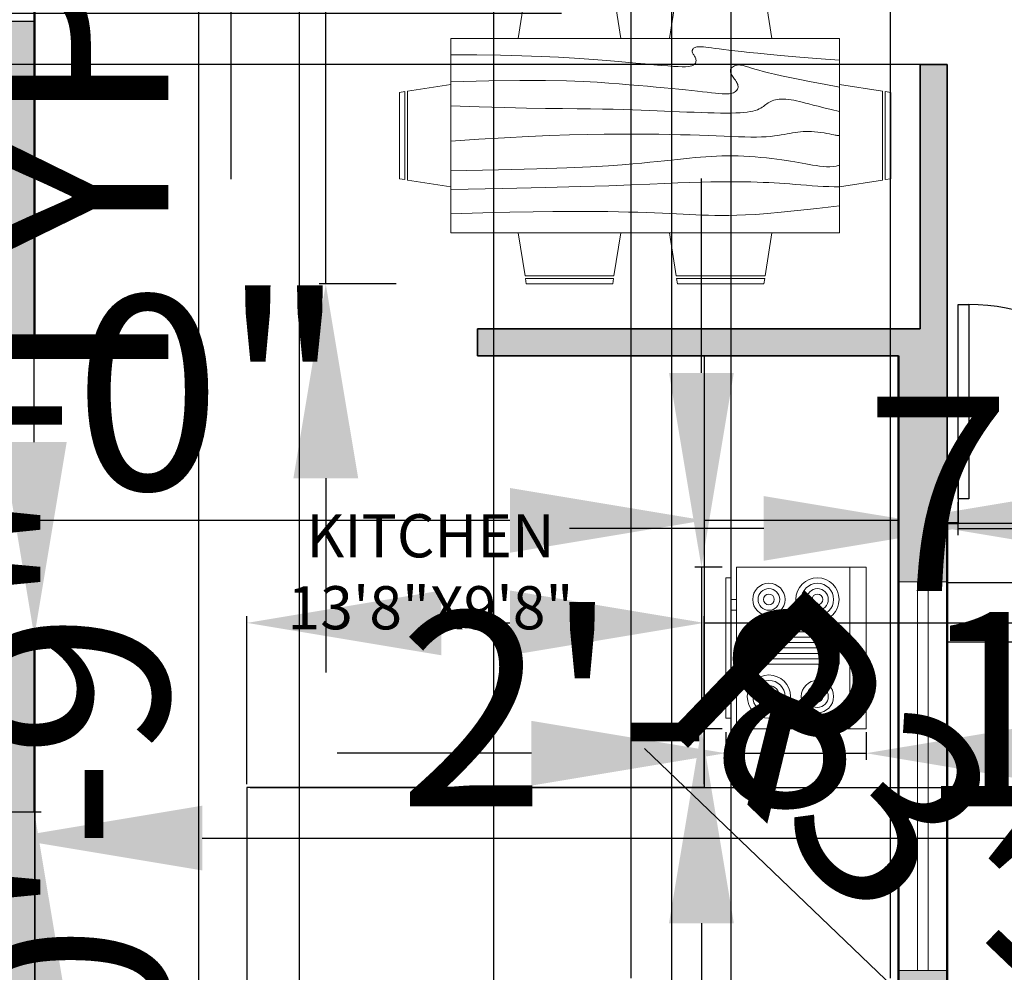
# Model space of a CAD drawing. Units: inches. Extents: x -299 to 1164, y -2 to 940.
# Tile 5 of 11: x 414 to 597, y 313 to 490. Entities that reach past the tile are written whole.
import ezdxf

# ---------------------------------------------------------------- set-up
doc = ezdxf.new("R2010")
doc.units = ezdxf.units.IN
for name, color, linetype, lineweight in [('A-AREA-IDEN', 3, 'Continuous', 25), ('A-EQPM', 8, 'Continuous', 18), ('A-FLOR-CASE', 7, 'Continuous', 25), ('A-FURN', 8, 'Continuous', 18), ('dimensions', 191, 'Continuous', 18), ('doors', 20, 'Continuous', 25), ('inner walls', 7, 'Continuous', 35), ('outer walls', 7, 'Continuous', 50), ('stairs', 6, 'Continuous', 25), ('windows', 130, 'Continuous', 18)]:
    doc.layers.add(name, color=color, linetype=linetype, lineweight=lineweight)
doc.layers.add('A-WALL-PATT', color=240, linetype='Continuous', lineweight=13, true_color=0xed1f24)
doc.styles.get("Standard").update_dxf_attribs({"font": 'arial.ttf'})
doc.dimstyles.new('ISO-25', dxfattribs={"dimtxt": 36, "dimasz": 36, "dimexe": 1.25, "dimexo": 0.625, "dimtad": 1, "dimlunit": 3, "dimtxsty": 'Standard', "dimcen": 2.5, "dimazin": 0, "dimtfac": 1, "dimtmove": 0, "dimatfit": 3, "dimfxl": 1, "dimarcsym": 0})

# ---------------------------------------------------------------- blocks, each defined once
blk = doc.blocks.new('Dining Set - 36 x 72 in.')
for p, q in [((-22, 27.5), (-22.1562, 26.50042)), ((-22, 27.5), (-6, 27.5)), ((-5.8437, 26.49966), (-6, 27.5)), ((6, 27.5), (5.8438, 26.50042)), ((6, 27.5), (22, 27.5)), ((22.1563, 26.49966), (22, 27.5)), ((-22.2343, 26.00059), (-23.4847, 17.99762)), ((-22.2304, 26), (-5.7608, 26)), ((-5.8416, 26.5), (-22.1534, 26.5)), ((-4.5152, 17.99762), (-5.7655, 25.99926)), ((5.7657, 26.00059), (4.5153, 17.99762)), ((5.7696, 26), (22.2392, 26)), ((22.1584, 26.5), (5.8466, 26.5)), ((23.4848, 17.99762), (22.2345, 25.99926)), ((36, 18), (-36, 18)), ((-36, 18), (-36, -18)), ((36, -18), (36, 18)), ((-44.0006, 8.23428), (-35.9976, 9.48474)), ((44.0006, 8.23428), (35.9976, 9.48474)), ((-45.5, 8), (-44.5004, 8.15617)), ((-45.5, 8), (-45.5, -8)), ((-44.5, -8.15843), (-44.5, 8.15338)), ((-44, 8.23041), (-44, -8.23915)), ((44, 8.23041), (44, -8.23915)), ((44.5, -8.15843), (44.5, 8.15338)), ((45.5, 8), (44.5005, 8.15617)), ((45.5, 8), (45.5, -8)), ((-44.4997, -8.15631), (-45.5, -8)), ((-35.9976, -9.48476), (-43.9993, -8.2345)), ((35.9976, -9.48476), (43.9993, -8.2345)), ((44.4997, -8.15631), (45.5, -8)), ((-36, -18), (36, -18)), ((-22.2343, -26.0006), (-23.4847, -17.99762)), ((-4.5152, -17.99762), (-5.7655, -25.99928)), ((5.7657, -26.0006), (4.5153, -17.99762)), ((23.4848, -17.99762), (22.2345, -25.99928)), ((-22.2304, -26), (-5.7608, -26)), ((-22, -27.5), (-22.1562, -26.50044)), ((-5.8416, -26.5), (-22.1534, -26.5)), ((-5.8437, -26.49967), (-6, -27.5)), ((5.7696, -26), (22.2392, -26)), ((6, -27.5), (5.8438, -26.50044)), ((22.1584, -26.5), (5.8466, -26.5)), ((22.1563, -26.49967), (22, -27.5)), ((-22, -27.5), (-6, -27.5)), ((6, -27.5), (22, -27.5))]:
    blk.add_line(p, q)
for points in [[(-36, 15), (-31.1772, 14.97754), (-26.8079, 14.91406), (-22.8538, 14.81543), (-19.276, 14.6875), (-16.0362, 14.53613), (-13.0957, 14.36718), (-10.4159, 14.18652), (-7.9583, 14), (-5.6904, 13.81315), (-3.6035, 13.63021), (-1.6954, 13.45508), (0.0365, 13.29166), (1.5945, 13.14388), (2.9811, 13.01562), (4.1988, 12.9108), (5.25, 12.83333), (6.1393, 12.78613), (6.8802, 12.76823), (7.4883, 12.77767), (7.9792, 12.8125), (8.3685, 12.87077), (8.6719, 12.95052), (8.9049, 13.0498), (9.0833, 13.16666), (9.2205, 13.29899), (9.3216, 13.44401), (9.3895, 13.59879), (9.4271, 13.76041), (9.4373, 13.92594), (9.4232, 14.09245), (9.3875, 14.257), (9.3333, 14.41666), (9.2638, 14.56917), (9.1836, 14.71484), (9.0975, 14.85465), (9.0104, 14.98958), (8.9272, 15.1206), (8.8529, 15.2487), (8.7922, 15.37483), (8.75, 15.5), (8.7305, 15.62467), (8.7344, 15.74739), (8.7617, 15.86621), (8.8125, 15.97916), (8.8867, 16.08431), (8.9844, 16.17968), (9.1055, 16.26334), (9.25, 16.33333), (9.4189, 16.38802), (9.6172, 16.42708), (9.8506, 16.45052), (10.125, 16.45833), (10.4463, 16.45052), (10.8203, 16.42708), (11.2529, 16.38802), (11.75, 16.33333), (12.3184, 16.26318), (12.9694, 16.17838), (13.7151, 16.07991), (14.5677, 15.96875), (15.5395, 15.84586), (16.6426, 15.71224), (17.8893, 15.56884), (19.2917, 15.41666), (20.859, 15.25667), (22.5879, 15.08984), (24.4721, 14.91715), (26.5052, 14.73958), (28.6809, 14.5581), (30.9929, 14.3737), (33.4347, 14.18733), (36, 14)], [(-36, 10), (-28.9766, 10.14274), (-23.1725, 10.20442), (-18.4241, 10.19775), (-14.5677, 10.13541), (-11.4399, 10.03011), (-8.877, 9.89453), (-6.7154, 9.74137), (-4.7917, 9.58333), (-2.9698, 9.43082), (-1.2246, 9.28515), (0.4415, 9.14534), (2.026, 9.01041), (3.5266, 8.87939), (4.9408, 8.7513), (6.266, 8.62516), (7.5, 8.5), (8.6411, 8.37549), (9.6914, 8.2539), (10.6538, 8.13818), (11.5312, 8.03125), (12.3267, 7.93603), (13.043, 7.85547), (13.6831, 7.79248), (14.25, 7.75), (14.7471, 7.7303), (15.1797, 7.73307), (15.5537, 7.75732), (15.875, 7.80208), (16.1494, 7.86637), (16.3828, 7.94922), (16.5811, 8.04964), (16.75, 8.16666), (16.8944, 8.29915), (17.0143, 8.44531), (17.1089, 8.60319), (17.1771, 8.77083), (17.218, 8.94629), (17.2305, 9.1276), (17.2137, 9.31282), (17.1667, 9.5), (17.0895, 9.6875), (16.987, 9.875), (16.8649, 10.0625), (16.7292, 10.25), (16.5856, 10.4375), (16.4401, 10.625), (16.2985, 10.8125), (16.1667, 11), (16.05, 11.18733), (15.9518, 11.3737), (15.8752, 11.5581), (15.8229, 11.73958), (15.798, 11.91715), (15.8034, 12.08984), (15.842, 12.25667), (15.9167, 12.41666), (16.0295, 12.56836), (16.1784, 12.70833), (16.3605, 12.83268), (16.5729, 12.9375), (16.8127, 13.01888), (17.0768, 13.07291), (17.3625, 13.0957), (17.6667, 13.08333), (17.9894, 13.03312), (18.3418, 12.94726), (18.7382, 12.82918), (19.1927, 12.68229), (19.7195, 12.51001), (20.3327, 12.31575), (21.0465, 12.10294), (21.875, 11.875), (22.8357, 11.63354), (23.959, 11.37304), (25.2786, 11.08618), (26.8282, 10.76562), (28.6414, 10.40405), (30.752, 9.99414), (33.1936, 9.52856), (36, 9)], [(-36, 5.5), (-30.7157, 5.3348), (-26.069, 5.20963), (-21.9946, 5.11767), (-18.4271, 5.05208), (-15.3009, 5.00602), (-12.5508, 4.97265), (-10.1112, 4.94515), (-7.9167, 4.91666), (-5.909, 4.88167), (-4.0586, 4.83984), (-2.3429, 4.79215), (-0.7396, 4.73958), (0.7739, 4.6831), (2.22, 4.6237), (3.6213, 4.56233), (5, 4.5), (6.373, 4.43782), (7.7344, 4.3776), (9.0723, 4.32129), (10.375, 4.27083), (11.6309, 4.22819), (12.8281, 4.19531), (13.9551, 4.17415), (15, 4.16666), (15.954, 4.17448), (16.819, 4.19791), (17.6001, 4.23698), (18.3021, 4.29166), (18.9299, 4.36198), (19.4883, 4.44791), (19.9823, 4.54948), (20.4167, 4.66666), (20.7969, 4.79899), (21.1302, 4.94401), (21.4245, 5.09879), (21.6875, 5.26041), (21.9271, 5.42594), (22.1511, 5.59245), (22.3672, 5.757), (22.5834, 5.91666), (22.8065, 6.06868), (23.0404, 6.21093), (23.2879, 6.34147), (23.5521, 6.45833), (23.8358, 6.55957), (24.142, 6.64323), (24.4735, 6.70735), (24.8334, 6.75), (25.2235, 6.76969), (25.642, 6.76692), (26.0858, 6.74267), (26.5521, 6.69791), (27.0379, 6.63362), (27.5404, 6.55078), (28.0565, 6.45036), (28.5834, 6.33333), (29.1242, 6.19987), (29.7071, 6.04687), (30.3661, 5.87044), (31.1354, 5.66666), (32.0493, 5.43164), (33.142, 5.16146), (34.4475, 4.85221), (36, 4.5)], [(-36, -1), (-30.7915, -0.6591), (-26.0195, -0.38216), (-21.6519, -0.16284), (-17.6563, 0.00521), (-14.0005, 0.12833), (-10.6523, 0.21289), (-7.5796, 0.26522), (-4.75, 0.29166), (-2.134, 0.29793), (0.2878, 0.28711), (2.5317, 0.26163), (4.6146, 0.22396), (6.5529, 0.17651), (8.3633, 0.12174), (10.0623, 0.06209), (11.6667, 0), (13.1899, -0.06201), (14.6341, -0.1211), (15.9982, -0.17432), (17.2813, -0.21875), (18.4823, -0.25147), (19.6003, -0.26953), (20.6343, -0.27002), (21.5834, -0.25), (22.4481, -0.20768), (23.2357, -0.14584), (23.9549, -0.06836), (24.6146, 0.02083), (25.2235, 0.11784), (25.7904, 0.21875), (26.3241, 0.31966), (26.8334, 0.41666), (27.3265, 0.50618), (27.8099, 0.58593), (28.2894, 0.65397), (28.7709, 0.70833), (29.2601, 0.74707), (29.763, 0.76823), (30.2855, 0.76985), (30.8334, 0.75), (31.4088, 0.70784), (31.9994, 0.64713), (32.589, 0.57275), (33.1615, 0.48958), (33.7008, 0.4025), (34.1908, 0.3164), (34.6153, 0.23616), (34.9584, 0.16666), (35.2099, 0.11165), (35.3848, 0.07031), (35.504, 0.04069), (35.5886, 0.02083), (35.6594, 0.00879), (35.7377, 0.0026), (35.8442, 0.00032), (36, 0)], [(-36, -6.5), (-27.1843, -6.31267), (-20.084, -6.1263), (-14.469, -5.9419), (-10.1094, -5.76042), (-6.7752, -5.58285), (-4.2363, -5.41016), (-2.2629, -5.24333), (-0.625, -5.08334), (0.8708, -4.93099), (2.2715, -4.78646), (3.5872, -4.64974), (4.8281, -4.52084), (6.0046, -4.39974), (7.127, -4.28646), (8.2053, -4.18099), (9.25, -4.08334), (10.2705, -3.99382), (11.2734, -3.91407), (12.2647, -3.84603), (13.25, -3.79167), (14.2354, -3.75293), (15.2266, -3.73177), (16.2295, -3.73015), (17.25, -3.75), (18.2912, -3.79248), (19.3451, -3.85547), (20.4009, -3.93604), (21.4479, -4.03125), (22.4754, -4.13819), (23.4727, -4.25391), (24.4289, -4.37549), (25.3334, -4.5), (26.1785, -4.62492), (26.9694, -4.74935), (27.7145, -4.87281), (28.4219, -4.99479), (29.1, -5.11483), (29.7572, -5.23242), (30.4016, -5.34709), (31.0417, -5.45834), (31.6837, -5.56437), (32.3262, -5.65821), (32.9658, -5.73153), (33.599, -5.77604), (34.2224, -5.78345), (34.8327, -5.74545), (35.4264, -5.65373), (36, -5.5)], [(-36, -10), (-26.4022, -9.81299), (-18.4675, -9.62891), (-11.9839, -9.45069), (-6.7396, -9.28125), (-2.5226, -9.12354), (0.8789, -8.98047), (3.6769, -8.85498), (6.0833, -8.75), (8.2767, -8.66765), (10.3021, -8.60677), (12.1712, -8.56543), (13.8958, -8.54167), (15.4876, -8.53353), (16.9583, -8.53907), (18.3197, -8.55632), (19.5834, -8.58334), (20.7616, -8.61841), (21.8685, -8.66081), (22.9188, -8.71004), (23.9271, -8.76563), (24.9081, -8.82707), (25.8763, -8.89388), (26.8465, -8.96558), (27.8334, -9.04167), (28.8474, -9.12118), (29.8828, -9.20117), (30.93, -9.27824), (31.9792, -9.34896), (33.0205, -9.40991), (34.0443, -9.45768), (35.0407, -9.48885), (36, -9.5)], [(-36, -14.5), (-30.0881, -14.33513), (-25.0332, -14.21224), (-20.7312, -14.12647), (-17.0781, -14.07292), (-13.97, -14.04671), (-11.3027, -14.04297), (-8.9724, -14.05681), (-6.875, -14.08334), (-4.9224, -14.11833), (-3.0905, -14.16016), (-1.3709, -14.20785), (0.2448, -14.26042), (1.7647, -14.3169), (3.1973, -14.3763), (4.5507, -14.43767), (5.8333, -14.5), (7.0554, -14.5621), (8.235, -14.62175), (9.3922, -14.67652), (10.5469, -14.72396), (11.7192, -14.76164), (12.929, -14.78711), (14.1965, -14.79794), (15.5417, -14.79167), (16.9933, -14.76424), (18.6152, -14.70508), (20.4804, -14.60197), (22.6615, -14.44271), (25.2312, -14.21509), (28.2624, -13.9069), (31.8277, -13.50594), (36, -13)]]:
    blk.add_lwpolyline(points)
blk = doc.blocks.new('Range-Oven - 30 in top')
for p, q in [((0, -3), (30, -3)), ((12, -6), (18, -6)), ((13, -20), (13, -6)), ((14, -6), (14, -20)), ((15, -20), (15, -6)), ((16, -6), (16, -20)), ((17, -20), (17, -6)), ((18, -20), (12, -20)), ((6, -24), (6, -25)), ((8, -25), (8, -24)), ((22, -25), (22, -24)), ((24, -24), (24, -25))]:
    blk.add_line(p, q)
for points in [[(0, -24), (0, 0), (30, 0), (30, -24)], [(12, -21), (12, -5), (18, -5), (18, -21)], [(2, -26), (2, -25), (28, -25), (28, -26)]]:
    blk.add_lwpolyline(points, close=True)
for centre, radius in [((6, -9), 4), ((6, -9), 3), ((6, -9), 2), ((24, -9), 3), ((24, -9), 2), ((6, -9), 1), ((24, -9), 1), ((24, -18), 4), ((6, -18), 3), ((6, -18), 2), ((24, -18), 3), ((24, -18), 2), ((6, -18), 1), ((24, -18), 1)]:
    blk.add_circle(centre, radius)
blk = doc.blocks.new('WIN-72IN')
for p, q in [((0, 5.5), (72, 5.5)), ((0, 3.5), (72, 3.5))]:
    blk.add_line(p, q)
blk.add_lwpolyline([(0, 0), (72, 0), (72, 9), (0, 9)], close=True)
blk = doc.blocks.new('DOOR-36IN')
blk.add_lwpolyline([(0, 36), (2, 36), (2, 0), (0, 0)], close=True)
blk.add_arc((2.32, 2.25), 33.75, 356.1776, 90.5492)
blk = doc.blocks.new('*D25')
at = {"layer": 'Defpoints', "color": 0, "transparency": 16777216}
for p in [(443.65, 597.1), (453.38, 597.1), (443.65, 532.21)]:
    blk.add_point(p, dxfattribs=at)
at = {"layer": 'dimensions', "color": 0, "lineweight": -2, "transparency": 16777216}
for p, q in [((453.38, 633.1), (453.38, 916.77)), ((444.27, 597.1), (454.63, 597.1)), ((453.38, 532.21), (453.38, 597.1)), ((444.27, 532.21), (454.63, 532.21)), ((453.38, 496.21), (453.38, 460.21))]:
    blk.add_line(p, q, dxfattribs=at)
at = {"layer": 'dimensions', "color": 0, "transparency": 16777216}
for points in [[(447.38, 633.1), (459.38, 633.1), (453.38, 597.1)], [(447.38, 496.21), (459.38, 496.21), (453.38, 532.21)]]:
    blk.add_solid(points, dxfattribs=at)
at = {"layer": 'dimensions', "color": 0, "transparency": 16777216, "insert": (434.13, 792.94), "char_height": 36, "attachment_point": 5, "rotation": 90}
blk.add_mtext('SOFA 5\'-5"', dxfattribs=at)
blk = doc.blocks.new('*D27')
at = {"layer": 'Defpoints', "color": 0, "transparency": 16777216}
for p in [(412.07, 375.49), (416.95, 375.49), (412.07, 342.99)]:
    blk.add_point(p, dxfattribs=at)
at = {"layer": 'dimensions', "color": 0, "lineweight": -2, "transparency": 16777216}
for p, q in [((416.95, 411.49), (416.95, 915.12)), ((412.7, 375.49), (418.2, 375.49)), ((416.95, 342.99), (416.95, 375.49)), ((412.7, 342.99), (418.2, 342.99)), ((416.95, 306.99), (416.95, 270.99))]:
    blk.add_line(p, q, dxfattribs=at)
at = {"layer": 'dimensions', "color": 0, "transparency": 16777216}
for points in [[(410.95, 411.49), (422.95, 411.49), (416.95, 375.49)], [(410.95, 306.99), (422.95, 306.99), (416.95, 342.99)]]:
    blk.add_solid(points, dxfattribs=at)
at = {"layer": 'dimensions', "color": 0, "transparency": 16777216, "insert": (397.69, 681.3), "char_height": 36, "attachment_point": 5, "rotation": 90}
blk.add_mtext('DOOR 2\'-8 1/2" TYP.', dxfattribs=at)
blk = doc.blocks.new('*D28')
at = {"layer": 'Defpoints', "color": 0, "transparency": 16777216}
for p in [(379.74, 342.99), (412.07, 342.99), (412.07, 338.11)]:
    blk.add_point(p, dxfattribs=at)
at = {"layer": 'dimensions', "color": 0, "lineweight": -2, "transparency": 16777216}
for p, q in [((379.74, 342.36), (379.74, 336.86)), ((412.07, 342.36), (412.07, 336.86)), ((343.74, 338.11), (307.74, 338.11)), ((379.74, 338.11), (412.07, 338.11)), ((448.07, 338.11), (789.26, 338.11))]:
    blk.add_line(p, q, dxfattribs=at)
at = {"layer": 'dimensions', "color": 0, "transparency": 16777216}
for points in [[(343.74, 344.11), (343.74, 332.11), (379.74, 338.11)], [(448.07, 344.11), (448.07, 332.11), (412.07, 338.11)]]:
    blk.add_solid(points, dxfattribs=at)
at = {"layer": 'dimensions', "color": 0, "transparency": 16777216, "insert": (636.66, 357.35), "char_height": 36, "attachment_point": 5}
blk.add_mtext('2\'-8 1/2" TYP.', dxfattribs=at)
blk = doc.blocks.new('*D30')
at = {"layer": 'Defpoints', "color": 0, "transparency": 16777216}
for p in [(376.07, 192.49), (386.87, 192.49), (376.07, 183.49)]:
    blk.add_point(p, dxfattribs=at)
at = {"layer": 'dimensions', "color": 0, "lineweight": -2, "transparency": 16777216}
for p, q in [((386.87, 228.49), (386.87, 485.18)), ((376.7, 192.49), (388.12, 192.49)), ((386.87, 183.49), (386.87, 192.49)), ((376.7, 183.49), (388.12, 183.49)), ((386.87, 147.49), (386.87, 111.49))]:
    blk.add_line(p, q, dxfattribs=at)
at = {"layer": 'dimensions', "color": 0, "transparency": 16777216}
for points in [[(380.87, 228.49), (392.87, 228.49), (386.87, 192.49)], [(380.87, 147.49), (392.87, 147.49), (386.87, 183.49)]]:
    blk.add_solid(points, dxfattribs=at)
at = {"layer": 'dimensions', "color": 0, "transparency": 16777216, "insert": (367.87, 374.83), "char_height": 36, "attachment_point": 5, "rotation": 90}
blk.add_mtext('0\'-9" TYP.', dxfattribs=at)
blk = doc.blocks.new('*D34')
at = {"layer": 'Defpoints', "color": 0, "transparency": 16777216}
for p in [(443.84, 222.49), (447.44, 222.49), (443.84, 213.49)]:
    blk.add_point(p, dxfattribs=at)
at = {"layer": 'dimensions', "color": 0, "lineweight": -2, "transparency": 16777216}
for p, q in [((447.44, 258.49), (447.44, 515.18)), ((444.47, 222.49), (448.69, 222.49)), ((447.44, 213.49), (447.44, 222.49)), ((444.47, 213.49), (448.69, 213.49)), ((447.44, 177.49), (447.44, 141.49))]:
    blk.add_line(p, q, dxfattribs=at)
at = {"layer": 'dimensions', "color": 0, "transparency": 16777216}
for points in [[(441.44, 258.49), (453.44, 258.49), (447.44, 222.49)], [(441.44, 177.49), (453.44, 177.49), (447.44, 213.49)]]:
    blk.add_solid(points, dxfattribs=at)
at = {"layer": 'dimensions', "color": 0, "transparency": 16777216, "insert": (428.44, 404.83), "char_height": 36, "attachment_point": 5, "rotation": 90}
blk.add_mtext('0\'-9" TYP.', dxfattribs=at)
blk = doc.blocks.new('*D35')
at = {"layer": 'Defpoints', "color": 0, "transparency": 16777216}
for p in [(307.07, 495.34), (268.07, 489.49), (307.07, 489.49)]:
    blk.add_point(p, dxfattribs=at)
at = {"layer": 'dimensions', "color": 0, "lineweight": -2, "transparency": 16777216}
for p, q in [((268.07, 490.11), (268.07, 496.59)), ((307.07, 490.11), (307.07, 496.59)), ((232.07, 495.34), (196.07, 495.34)), ((268.07, 495.34), (307.07, 495.34)), ((343.07, 495.34), (749.73, 495.34))]:
    blk.add_line(p, q, dxfattribs=at)
at = {"layer": 'dimensions', "color": 0, "transparency": 16777216}
for points in [[(232.07, 501.34), (232.07, 489.34), (268.07, 495.34)], [(343.07, 501.34), (343.07, 489.34), (307.07, 495.34)]]:
    blk.add_solid(points, dxfattribs=at)
at = {"layer": 'dimensions', "color": 0, "transparency": 16777216, "insert": (564.4, 514.36), "char_height": 36, "attachment_point": 5}
blk.add_mtext('VENT 3\'-3" TYP.', dxfattribs=at)
blk = doc.blocks.new('*D37')
at = {"layer": 'Defpoints', "color": 0, "transparency": 16777216}
for p in [(588.07, 400.99), (624.7, 400.99), (624.7, 395.5)]:
    blk.add_point(p, dxfattribs=at)
at = {"layer": 'dimensions', "color": 0, "lineweight": -2, "transparency": 16777216}
for p, q in [((588.07, 400.36), (588.07, 394.25)), ((624.7, 400.36), (624.7, 394.25)), ((552.07, 395.5), (516.07, 395.5)), ((588.07, 395.5), (624.7, 395.5)), ((660.7, 395.5), (1164.33, 395.5))]:
    blk.add_line(p, q, dxfattribs=at)
at = {"layer": 'dimensions', "color": 0, "transparency": 16777216}
for points in [[(552.07, 401.5), (552.07, 389.5), (588.07, 395.5)], [(660.7, 401.5), (660.7, 389.5), (624.7, 395.5)]]:
    blk.add_solid(points, dxfattribs=at)
at = {"layer": 'dimensions', "color": 0, "transparency": 16777216, "insert": (930.51, 414.76), "char_height": 36, "attachment_point": 5}
blk.add_mtext('DOOR 3\'-0 1/2" TYP.', dxfattribs=at)
blk = doc.blocks.new('*D38')
at = {"layer": 'Defpoints', "color": 0, "transparency": 16777216}
for p in [(624.7, 437.08), (630.19, 437.08), (624.7, 400.99)]:
    blk.add_point(p, dxfattribs=at)
at = {"layer": 'dimensions', "color": 0, "lineweight": -2, "transparency": 16777216}
for p, q in [((630.19, 473.08), (630.19, 729.74)), ((625.32, 437.08), (631.44, 437.08)), ((630.19, 400.99), (630.19, 437.08)), ((625.32, 400.99), (631.44, 400.99)), ((630.19, 364.99), (630.19, 328.99))]:
    blk.add_line(p, q, dxfattribs=at)
at = {"layer": 'dimensions', "color": 0, "transparency": 16777216}
for points in [[(624.19, 473.08), (636.19, 473.08), (630.19, 437.08)], [(624.19, 364.99), (636.19, 364.99), (630.19, 400.99)]]:
    blk.add_solid(points, dxfattribs=at)
at = {"layer": 'dimensions', "color": 0, "transparency": 16777216, "insert": (611.17, 619.41), "char_height": 36, "attachment_point": 5, "rotation": 90}
blk.add_mtext('3\'-0" TYP.', dxfattribs=at)
blk = doc.blocks.new('*D39')
at = {"layer": 'Defpoints', "color": 0, "transparency": 16777216}
for p in [(575.6, 509.45), (484.6, 495.8), (575.6, 495.8)]:
    blk.add_point(p, dxfattribs=at)
at = {"layer": 'dimensions', "color": 0, "lineweight": -2, "transparency": 16777216}
for p, q in [((484.6, 496.43), (484.6, 510.7)), ((520.6, 509.45), (539.6, 509.45)), ((575.6, 496.43), (575.6, 510.7)), ((575.6, 509.45), (1008.53, 509.45))]:
    blk.add_line(p, q, dxfattribs=at)
at = {"layer": 'dimensions', "color": 0, "transparency": 16777216}
for points in [[(520.6, 515.45), (520.6, 503.45), (484.6, 509.45)], [(539.6, 515.45), (539.6, 503.45), (575.6, 509.45)]]:
    blk.add_solid(points, dxfattribs=at)
at = {"layer": 'dimensions', "color": 0, "transparency": 16777216, "insert": (810.07, 528.69), "char_height": 36, "attachment_point": 5}
blk.add_mtext('DINING SET 7\'-7"', dxfattribs=at)
blk = doc.blocks.new('*D40')
at = {"layer": 'Defpoints', "color": 0, "transparency": 16777216}
for p in [(470.95, 495.8), (484.6, 495.8), (484.6, 440.8)]:
    blk.add_point(p, dxfattribs=at)
at = {"layer": 'dimensions', "color": 0, "lineweight": -2, "transparency": 16777216}
for p, q in [((470.95, 531.8), (470.95, 666.2)), ((483.98, 495.8), (469.7, 495.8)), ((470.95, 440.8), (470.95, 495.8)), ((483.98, 440.8), (469.7, 440.8)), ((470.95, 404.8), (470.95, 368.8))]:
    blk.add_line(p, q, dxfattribs=at)
at = {"layer": 'dimensions', "color": 0, "transparency": 16777216}
for points in [[(464.95, 531.8), (476.95, 531.8), (470.95, 495.8)], [(464.95, 404.8), (476.95, 404.8), (470.95, 440.8)]]:
    blk.add_solid(points, dxfattribs=at)
at = {"layer": 'dimensions', "color": 0, "transparency": 16777216, "insert": (452.33, 617), "char_height": 36, "attachment_point": 5, "rotation": 90}
blk.add_mtext('4\'-7"', dxfattribs=at)
blk = doc.blocks.new('*D41')
at = {"layer": 'Defpoints', "color": 0, "transparency": 16777216}
for p in [(545.04, 388.33), (540.54, 358.33), (545.04, 358.33)]:
    blk.add_point(p, dxfattribs=at)
at = {"layer": 'dimensions', "color": 0, "lineweight": -2, "transparency": 16777216}
for p, q in [((540.54, 424.33), (540.54, 460.33)), ((544.41, 388.33), (539.29, 388.33)), ((540.54, 388.33), (540.54, 358.33)), ((544.41, 358.33), (539.29, 358.33)), ((540.54, 322.33), (540.54, -1.56))]:
    blk.add_line(p, q, dxfattribs=at)
at = {"layer": 'dimensions', "color": 0, "transparency": 16777216}
for points in [[(534.54, 424.33), (546.54, 424.33), (540.54, 388.33)], [(534.54, 322.33), (546.54, 322.33), (540.54, 358.33)]]:
    blk.add_solid(points, dxfattribs=at)
at = {"layer": 'dimensions', "color": 0, "transparency": 16777216, "insert": (521.3, 142.39), "char_height": 36, "attachment_point": 5, "rotation": 90}
blk.add_mtext('RANGE 2\'-6"', dxfattribs=at)
blk = doc.blocks.new('*D42')
at = {"layer": 'Defpoints', "color": 0, "transparency": 16777216}
for p in [(545.04, 358.33), (571.04, 358.33), (571.04, 353.83)]:
    blk.add_point(p, dxfattribs=at)
at = {"layer": 'dimensions', "color": 0, "lineweight": -2, "transparency": 16777216}
for p, q in [((545.04, 357.71), (545.04, 352.58)), ((571.04, 357.71), (571.04, 352.58)), ((509.04, 353.83), (473.04, 353.83)), ((545.04, 353.83), (571.04, 353.83)), ((607.04, 353.83), (740.6, 353.83))]:
    blk.add_line(p, q, dxfattribs=at)
at = {"layer": 'dimensions', "color": 0, "transparency": 16777216}
for points in [[(509.04, 359.83), (509.04, 347.83), (545.04, 353.83)], [(607.04, 359.83), (607.04, 347.83), (571.04, 353.83)]]:
    blk.add_solid(points, dxfattribs=at)
at = {"layer": 'dimensions', "color": 0, "transparency": 16777216, "insert": (691.82, 372.53), "char_height": 36, "attachment_point": 5}
blk.add_mtext('2\'-2"', dxfattribs=at)
blk = doc.blocks.new('*D46')
at = {"layer": 'Defpoints', "color": 0, "transparency": 16777216}
for p in [(579.07, 302.49), (770.93, 302.49), (579.07, 222.49)]:
    blk.add_point(p, dxfattribs=at)
at = {"layer": 'dimensions', "color": 0, "lineweight": -2, "transparency": 16777216}
for p, q in [((770.93, 302.49), (770.93, 435.63)), ((579.7, 302.49), (772.18, 302.49)), ((770.93, 258.49), (770.93, 266.49)), ((579.7, 222.49), (772.18, 222.49))]:
    blk.add_line(p, q, dxfattribs=at)
at = {"layer": 'dimensions', "color": 0, "transparency": 16777216}
for points in [[(764.93, 266.49), (776.93, 266.49), (770.93, 302.49)], [(764.93, 258.49), (776.93, 258.49), (770.93, 222.49)]]:
    blk.add_solid(points, dxfattribs=at)
at = {"layer": 'dimensions', "color": 0, "transparency": 16777216, "insert": (751.92, 387.06), "char_height": 36, "attachment_point": 5, "rotation": 90}
blk.add_mtext('6\'-8"', dxfattribs=at)
blk = doc.blocks.new('*D47')
at = {"layer": 'Defpoints', "color": 0, "transparency": 16777216}
for p in [(502.07, 668.99), (466.07, 222.49), (502.07, 222.49)]:
    blk.add_point(p, dxfattribs=at)
at = {"layer": 'dimensions', "color": 0, "lineweight": -2, "transparency": 16777216}
for p, q in [((466.07, 223.11), (466.07, 670.24)), ((502.07, 223.11), (502.07, 670.24)), ((430.07, 668.99), (394.07, 668.99)), ((466.07, 668.99), (502.07, 668.99)), ((538.07, 668.99), (670.99, 668.99))]:
    blk.add_line(p, q, dxfattribs=at)
at = {"layer": 'dimensions', "color": 0, "transparency": 16777216}
for points in [[(430.07, 674.99), (430.07, 662.99), (466.07, 668.99)], [(538.07, 674.99), (538.07, 662.99), (502.07, 668.99)]]:
    blk.add_solid(points, dxfattribs=at)
at = {"layer": 'dimensions', "color": 0, "transparency": 16777216, "insert": (622.53, 688.01), "char_height": 36, "attachment_point": 5}
blk.add_mtext('3\'-0"', dxfattribs=at)
blk = doc.blocks.new('*D48')
at = {"layer": 'Defpoints', "color": 0, "transparency": 16777216}
for p in [(546.07, 668.99), (535.07, 222.49), (546.07, 222.49)]:
    blk.add_point(p, dxfattribs=at)
at = {"layer": 'dimensions', "color": 0, "lineweight": -2, "transparency": 16777216}
for p, q in [((535.07, 223.11), (535.07, 670.24)), ((546.07, 223.11), (546.07, 670.24)), ((499.07, 668.99), (463.07, 668.99)), ((535.07, 668.99), (546.07, 668.99)), ((582.07, 668.99), (742.99, 668.99))]:
    blk.add_line(p, q, dxfattribs=at)
at = {"layer": 'dimensions', "color": 0, "transparency": 16777216}
for points in [[(499.07, 674.99), (499.07, 662.99), (535.07, 668.99)], [(582.07, 674.99), (582.07, 662.99), (546.07, 668.99)]]:
    blk.add_solid(points, dxfattribs=at)
at = {"layer": 'dimensions', "color": 0, "transparency": 16777216, "insert": (680.53, 687.99), "char_height": 36, "attachment_point": 5}
blk.add_mtext('0\'-11"', dxfattribs=at)
blk = doc.blocks.new('*D52')
at = {"layer": 'Defpoints', "color": 0, "transparency": 16777216}
for p in [(575.54, 668.99), (527.54, 311.49), (575.54, 311.49)]:
    blk.add_point(p, dxfattribs=at)
at = {"layer": 'dimensions', "color": 0, "lineweight": -2, "transparency": 16777216}
for p, q in [((527.54, 312.11), (527.54, 670.24)), ((575.54, 312.11), (575.54, 670.24)), ((491.54, 668.99), (455.54, 668.99)), ((527.54, 668.99), (575.54, 668.99)), ((611.54, 668.99), (745.94, 668.99))]:
    blk.add_line(p, q, dxfattribs=at)
at = {"layer": 'dimensions', "color": 0, "transparency": 16777216}
for points in [[(491.54, 674.99), (491.54, 662.99), (527.54, 668.99)], [(611.54, 674.99), (611.54, 662.99), (575.54, 668.99)]]:
    blk.add_solid(points, dxfattribs=at)
at = {"layer": 'dimensions', "color": 0, "transparency": 16777216, "insert": (696.74, 687.99), "char_height": 36, "attachment_point": 5}
blk.add_mtext('4\'-0"', dxfattribs=at)
blk = doc.blocks.new('*D53')
at = {"layer": 'Defpoints', "color": 0, "transparency": 16777216}
for p in [(177.57, 553.49), (586.07, 553.49), (586.07, 481.49)]:
    blk.add_point(p, dxfattribs=at)
at = {"layer": 'dimensions', "color": 0, "lineweight": -2, "transparency": 16777216}
for p, q in [((177.57, 589.49), (177.57, 722.63)), ((585.45, 553.49), (176.32, 553.49)), ((177.57, 481.49), (177.57, 553.49)), ((585.45, 481.49), (176.32, 481.49)), ((177.57, 445.49), (177.57, 409.49))]:
    blk.add_line(p, q, dxfattribs=at)
at = {"layer": 'dimensions', "color": 0, "transparency": 16777216}
for points in [[(171.57, 589.49), (183.57, 589.49), (177.57, 553.49)], [(171.57, 445.49), (183.57, 445.49), (177.57, 481.49)]]:
    blk.add_solid(points, dxfattribs=at)
at = {"layer": 'dimensions', "color": 0, "transparency": 16777216, "insert": (158.57, 674.06), "char_height": 36, "attachment_point": 5, "rotation": 90}
blk.add_mtext('6\'-0"', dxfattribs=at)
blk = doc.blocks.new('*D54')
at = {"layer": 'Defpoints', "color": 0, "transparency": 16777216}
for p in [(345.07, 490.99), (312.07, 460.49), (345.07, 460.49)]:
    blk.add_point(p, dxfattribs=at)
at = {"layer": 'dimensions', "color": 0, "lineweight": -2, "transparency": 16777216}
for p, q in [((276.07, 490.99), (240.07, 490.99)), ((312.07, 461.11), (312.07, 492.24)), ((312.07, 490.99), (345.07, 490.99)), ((345.07, 461.11), (345.07, 492.24)), ((381.07, 490.99), (514.63, 490.99))]:
    blk.add_line(p, q, dxfattribs=at)
at = {"layer": 'dimensions', "color": 0, "transparency": 16777216}
for points in [[(276.07, 496.99), (276.07, 484.99), (312.07, 490.99)], [(381.07, 496.99), (381.07, 484.99), (345.07, 490.99)]]:
    blk.add_solid(points, dxfattribs=at)
at = {"layer": 'dimensions', "color": 0, "transparency": 16777216, "insert": (465.85, 509.99), "char_height": 36, "attachment_point": 5}
blk.add_mtext('2\'-9"', dxfattribs=at)
blk = doc.blocks.new('*D56')
at = {"layer": 'Defpoints', "color": 0, "transparency": 16777216}
for p in [(541.07, 377.99), (456.35, 347.49), (541.07, 347.49)]:
    blk.add_point(p, dxfattribs=at)
at = {"layer": 'dimensions', "color": 0, "lineweight": -2, "transparency": 16777216}
for p, q in [((456.35, 348.11), (456.35, 379.24)), ((492.35, 377.99), (505.07, 377.99)), ((541.07, 348.11), (541.07, 379.24)), ((541.07, 377.99), (757.61, 377.99))]:
    blk.add_line(p, q, dxfattribs=at)
at = {"layer": 'dimensions', "color": 0, "transparency": 16777216}
for points in [[(492.35, 383.99), (492.35, 371.99), (456.35, 377.99)], [(505.07, 383.99), (505.07, 371.99), (541.07, 377.99)]]:
    blk.add_solid(points, dxfattribs=at)
at = {"layer": 'dimensions', "color": 0, "transparency": 16777216, "insert": (667.34, 397.23), "char_height": 36, "attachment_point": 5}
blk.add_mtext('7\'-0 1/2"', dxfattribs=at)
blk = doc.blocks.new('*D57')
at = {"layer": 'Defpoints', "color": 0, "transparency": 16777216}
for p in [(541.07, 427.49), (577.07, 427.49), (541.07, 396.99)]:
    blk.add_point(p, dxfattribs=at)
at = {"layer": 'dimensions', "color": 0, "lineweight": -2, "transparency": 16777216}
for p, q in [((541.07, 426.86), (541.07, 395.74)), ((577.07, 426.86), (577.07, 395.74)), ((505.07, 396.99), (372.15, 396.99)), ((577.07, 396.99), (541.07, 396.99)), ((613.07, 396.99), (649.07, 396.99))]:
    blk.add_line(p, q, dxfattribs=at)
at = {"layer": 'dimensions', "color": 0, "transparency": 16777216}
for points in [[(505.07, 402.99), (505.07, 390.99), (541.07, 396.99)], [(613.07, 402.99), (613.07, 390.99), (577.07, 396.99)]]:
    blk.add_solid(points, dxfattribs=at)
at = {"layer": 'dimensions', "color": 0, "transparency": 16777216, "insert": (420.61, 416.01), "char_height": 36, "attachment_point": 5}
blk.add_mtext('3\'-0"', dxfattribs=at)
blk = doc.blocks.new('*D58')
at = {"layer": 'Defpoints', "color": 0, "transparency": 16777216}
for p in [(456.35, 347.49), (770.93, 347.49), (456.35, 311.49)]:
    blk.add_point(p, dxfattribs=at)
at = {"layer": 'dimensions', "color": 0, "lineweight": -2, "transparency": 16777216}
for p, q in [((770.93, 383.49), (770.93, 516.41)), ((456.97, 347.49), (772.18, 347.49)), ((770.93, 311.49), (770.93, 347.49)), ((456.97, 311.49), (772.18, 311.49)), ((770.93, 275.49), (770.93, 239.49))]:
    blk.add_line(p, q, dxfattribs=at)
at = {"layer": 'dimensions', "color": 0, "transparency": 16777216}
for points in [[(764.93, 383.49), (776.93, 383.49), (770.93, 347.49)], [(764.93, 275.49), (776.93, 275.49), (770.93, 311.49)]]:
    blk.add_solid(points, dxfattribs=at)
at = {"layer": 'dimensions', "color": 0, "transparency": 16777216, "insert": (751.91, 467.95), "char_height": 36, "attachment_point": 5, "rotation": 90}
blk.add_mtext('3\'-0"', dxfattribs=at)
blk = doc.blocks.new('*D59')
at = {"layer": 'Defpoints', "color": 0, "transparency": 16777216}
for p in [(697.05, 194.59), (730.81, 162.24)]:
    blk.add_point(p, dxfattribs=at)
at = {"layer": 'dimensions', "color": 0, "lineweight": -2, "transparency": 16777216}
for p, q in [((530.01, 354.68), (671.06, 219.5)), ((730.81, 162.24), (697.05, 194.59))]:
    blk.add_line(p, q, dxfattribs=at)
at = {"layer": 'dimensions', "color": 0, "transparency": 16777216}
blk.add_solid([(675.21, 223.83), (666.91, 215.17), (697.05, 194.59)], dxfattribs=at)
at = {"layer": 'dimensions', "color": 0, "transparency": 16777216, "insert": (600.7, 313.27), "char_height": 36, "attachment_point": 5, "rotation": 316.2186}
blk.add_mtext('R3\'-11"', dxfattribs=at)

msp = doc.modelspace()

# ---------------------------------------------------------------- hatches: boundary and pattern name
at = {"layer": 'A-WALL-PATT'}
h = msp.add_hatch(color=256, dxfattribs=at)
h.dxf.hatch_style = 1
h.paths.add_polyline_path([(312.071, 460.489), (307.071, 460.489), (307.071, 432.489), (307.071, 427.489), (372.071, 427.489), (372.071, 375.489), (372.071, 370.489), (380.071, 370.489, -0.0217424), (380.071, 372.989), (380.071, 375.489), (377.071, 375.489), (377.071, 427.489), (417.071, 427.489), (417.071, 489.489), (412.071, 489.489), (412.071, 484.489), (412.071, 432.489), (312.071, 432.489)], flags=17)
h.paths.add_polyline_path([(340.071, 372.989, -0.0217424), (340.071, 375.489), (268.071, 375.489), (268.071, 427.489), (268.071, 432.489), (268.071, 484.489), (268.071, 489.489), (268.071, 629.489), (412.071, 629.489), (412.071, 527.563, -0.0185322), (414.571, 527.489), (417.071, 527.489), (417.071, 629.489), (581.071, 629.489), (581.071, 553.489), (586.071, 553.489), (586.071, 629.489), (730.071, 629.489), (730.071, 405.489), (713.071, 405.489), (713.071, 396.489), (739.071, 396.489), (739.071, 638.489), (259.071, 638.489), (259.071, 183.489), (304.071, 183.489), (304.071, 192.489), (268.071, 192.489), (268.071, 370.489), (340.071, 370.489)])
h.paths.add_polyline_path([(417.071, 188.489), (417.071, 213.489), (461.071, 213.489), (461.071, 188.489)], flags=16)
h.paths.add_polyline_path([(586.071, 313.578), (577.071, 313.578), (577.071, 311.489), (575.54, 311.489), (575.54, 302.489), (586.071, 302.489)], flags=16)
h.paths.add_polyline_path([(586.071, 405.489), (586.071, 481.489), (581.071, 481.489), (581.071, 432.489), (499.071, 432.489), (499.071, 427.489), (577.071, 427.489), (577.071, 385.578), (586.071, 385.578), (586.071, 396.489)], flags=17)
h.paths.add_polyline_path([(641.071, 405.489), (624.071, 405.489, -0.0333689), (624.071, 400.989), (624.071, 396.489), (641.071, 396.489)], flags=17)
h.paths.add_polyline_path([(491.866, 222.489), (491.866, 213.489), (586.071, 213.489), (586.071, 222.489)])
edge = h.paths.add_edge_path()
edge.add_line((467.866, 213.489), (467.866, 222.489))
edge.add_line((467.866, 222.489), (466.071, 222.489))
edge.add_line((466.071, 222.489), (466.071, 302.489))
edge.add_line((466.071, 302.489), (527.54, 302.489))
edge.add_line((527.54, 302.489), (527.54, 311.489))
edge.add_line((527.54, 311.489), (449.071, 311.489))
edge.add_line((449.071, 311.489), (449.071, 308.989))
edge.add_arc((420.339, 307.739), 28.759, -2.4911, 2.4911, ccw=False)
edge.add_line((449.071, 306.489), (461.071, 306.489))
edge.add_line((461.071, 306.489), (461.071, 222.489))
edge.add_line((461.071, 222.489), (443.844, 222.489))
edge.add_line((443.844, 222.489), (443.844, 213.489))
edge.add_line((443.844, 213.489), (419.844, 213.489))
edge.add_line((419.844, 213.489), (419.844, 222.489))
edge.add_line((419.844, 222.489), (417.071, 222.489))
edge.add_line((417.071, 222.489), (417.071, 306.489))
edge.add_line((417.071, 306.489), (417.071, 311.489))
edge.add_line((417.071, 311.489), (417.071, 375.489))
edge.add_line((417.071, 375.489), (412.071, 375.489))
edge.add_line((412.071, 375.489), (412.071, 370.489))
edge.add_line((412.071, 370.489), (412.071, 192.489))
edge.add_line((412.071, 192.489), (376.071, 192.489))
edge.add_line((376.071, 192.489), (376.071, 183.489))
edge.add_line((376.071, 183.489), (412.071, 183.489))
edge.add_line((412.071, 183.489), (466.071, 183.489))
edge.add_line((466.071, 183.489), (466.071, 213.489))
edge.add_line((466.071, 213.489), (467.866, 213.489))

# ---------------------------------------------------------------- linework, layer by layer
at = {"layer": 'A-FLOR-CASE'}
for p, q in [((577.071, 427.489), (541.071, 427.489)), ((541.071, 427.489), (541.071, 347.489)), ((541.071, 347.489), (456.348, 347.489)), ((456.348, 347.489), (456.348, 311.489))]:
    msp.add_line(p, q, dxfattribs=at)
at = {"layer": 'doors'}
for p, q in [((412.071, 489.489), (417.071, 489.489)), ((586.071, 405.489), (586.071, 396.489)), ((588.071, 405.489), (588.071, 396.489))]:
    msp.add_line(p, q, dxfattribs=at)
at = {"layer": 'inner walls'}
for p, q in [((417.071, 491.489), (417.071, 427.489)), ((586.071, 481.489), (581.071, 481.489)), ((581.071, 481.489), (581.071, 432.489)), ((586.071, 481.489), (586.071, 405.489)), ((581.071, 432.489), (499.071, 432.489)), ((499.071, 432.489), (499.071, 427.489)), ((417.071, 427.489), (377.071, 427.489)), ((577.071, 427.489), (499.071, 427.489)), ((417.071, 375.489), (410.071, 375.489)), ((417.071, 375.489), (417.071, 311.489))]:
    msp.add_line(p, q, dxfattribs=at)
at = {"layer": 'outer walls'}
for p, q in [((577.071, 427.489), (577.071, 311.489)), ((588.071, 405.489), (586.071, 405.489)), ((586.071, 396.489), (586.071, 302.489)), ((588.071, 396.489), (586.071, 396.489))]:
    msp.add_line(p, q, dxfattribs=at)
at = {"layer": 'stairs'}
for p, q in [((588.071, 396.489), (624.071, 396.489)), ((586.071, 385.489), (624.071, 385.489)), ((586.071, 374.489), (624.071, 374.489))]:
    msp.add_line(p, q, dxfattribs=at)

# ---------------------------------------------------------------- block references
at = {"layer": 'A-EQPM', "rotation": 269.9999999999999}
msp.add_blockref('Range-Oven - 30 in top', (571.036, 388.335), dxfattribs=at)
at = {"layer": 'A-FURN'}
msp.add_blockref('Dining Set - 36 x 72 in.', (530.1, 468.3), dxfattribs=at)
at = {"layer": 'doors'}
msp.add_blockref('DOOR-36IN', (588.071, 400.989), dxfattribs=at)
at = {"layer": 'windows', "rotation": 270}
msp.add_blockref('WIN-72IN', (577.071, 385.578), dxfattribs=at)

# ---------------------------------------------------------------- texts
at = {"layer": 'A-AREA-IDEN', "insert": (455.421, 398.131), "char_height": 8, "attachment_point": 1}
msp.add_mtext_dynamic_manual_height_columns('\\pxqc,t15;KITCHEN\\P13\'8"X9\'8"', width=69.83809, gutter_width=12.5, heights=[0], dxfattribs=at)

# ---------------------------------------------------------------- dimensions: what is measured, and where the dimension line sits
at = {"layer": 'dimensions'}
for base, p1, p2, angle, text, picture, middle in [((453.378, 597.099), (443.646, 532.214), (443.646, 597.099), 90, 'SOFA <>', '*D25', (434.127, 792.936)), ((416.946, 375.489), (412.071, 342.989), (412.071, 375.489), 90, 'DOOR <> TYP.', '*D27', (397.695, 681.304)), ((630.192, 437.079), (624.698, 400.989), (624.698, 437.079), 90, '<> TYP.', '*D38', (611.174, 619.411)), ((447.444, 222.489), (443.844, 213.489), (443.844, 222.489), 90, '<> TYP.', '*D34', (428.438, 404.833)), ((386.871, 192.489), (376.071, 183.489), (376.071, 192.489), 90, '<> TYP.', '*D30', (367.865, 374.833)), ((540.536, 358.335), (545.036, 388.335), (545.036, 358.335), 270, 'RANGE <>', '*D41', (521.297, 142.385))]:
    dim = msp.add_linear_dim(base=base, p1=p1, p2=p2, angle=angle, text=text, dimstyle='ISO-25', override={"dimdec": 1, "dimlfac": 1, "dimrnd": 0, "dimzin": 1, "dimdsep": 46, "dimlunit": 4, "dimfrac": 2}, dxfattribs=at)
    dim.commit()
    dim.dimension.update_dxf_attribs({"geometry": picture, "text_midpoint": middle})
for base, p1, p2, angle, picture, middle in [((177.571, 553.489), (586.071, 481.489), (586.071, 553.489), 90, '*D53', (158.565, 674.061)), ((470.95, 495.8), (484.6, 440.8), (484.6, 495.8), 90, '*D40', (452.325, 616.998)), ((345.071, 490.989), (312.071, 460.489), (345.071, 460.489), 0.00004, '*D54', (465.852, 509.995)), ((770.929, 347.489), (456.348, 311.489), (456.348, 347.489), 90, '*D58', (751.911, 467.95)), ((541.071, 396.989), (577.071, 427.489), (541.071, 427.489), 180, '*D57', (420.61, 416.007)), ((770.929, 302.489), (579.071, 222.489), (579.071, 302.489), 90, '*D46', (751.923, 387.061))]:
    dim = msp.add_linear_dim(base=base, p1=p1, p2=p2, angle=angle, dimstyle='ISO-25', override={"dimdec": 1, "dimlfac": 1, "dimrnd": 0, "dimzin": 1, "dimdsep": 46, "dimlunit": 4, "dimfrac": 2}, dxfattribs=at)
    dim.commit()
    dim.dimension.update_dxf_attribs({"geometry": picture, "text_midpoint": middle})
for base, p1, p2, picture, middle in [((502.071, 668.989), (466.071, 222.489), (502.071, 222.489), '*D47', (622.532, 688.007)), ((575.54, 668.989), (527.54, 311.489), (575.54, 311.489), '*D52', (696.738, 687.995)), ((546.071, 668.989), (535.071, 222.489), (546.071, 222.489), '*D48', (680.53, 687.995)), ((541.071, 377.989), (456.348, 347.489), (541.071, 347.489), '*D56', (667.34, 397.228)), ((571.036, 353.835), (545.036, 358.335), (571.036, 358.335), '*D42', (691.817, 372.534))]:
    dim = msp.add_linear_dim(base=base, p1=p1, p2=p2, dimstyle='ISO-25', override={"dimdec": 1, "dimlfac": 1, "dimrnd": 0, "dimzin": 1, "dimdsep": 46, "dimlunit": 4, "dimfrac": 2}, dxfattribs=at)
    dim.commit()
    dim.dimension.update_dxf_attribs({"geometry": picture, "text_midpoint": middle})
for base, p1, p2, text, picture, middle in [((575.6, 509.45), (484.6, 495.8), (575.6, 495.8), 'DINING SET <>', '*D39', (810.066, 528.689)), ((307.071, 495.339), (268.071, 489.489), (307.071, 489.489), 'VENT <> TYP.', '*D35', (564.399, 514.357)), ((624.698, 395.495), (588.071, 400.989), (624.698, 400.989), 'DOOR <> TYP.', '*D37', (930.512, 414.759)), ((412.071, 338.114), (379.736, 342.989), (412.071, 342.989), '<> TYP.', '*D28', (636.665, 357.353))]:
    dim = msp.add_linear_dim(base=base, p1=p1, p2=p2, text=text, dimstyle='ISO-25', override={"dimdec": 1, "dimlfac": 1, "dimrnd": 0, "dimzin": 1, "dimdsep": 46, "dimlunit": 4, "dimfrac": 2}, dxfattribs=at)
    dim.commit()
    dim.dimension.update_dxf_attribs({"geometry": picture, "text_midpoint": middle})
dim = msp.add_radius_dim(center=(730.81, 162.239), mpoint=(697.053, 194.59), dimstyle='ISO-25', override={"dimdec": 1, "dimlfac": 1, "dimrnd": 0, "dimzin": 1, "dimdsep": 46, "dimlunit": 4, "dimfrac": 2}, dxfattribs=at)
dim.commit()
dim.dimension.update_dxf_attribs({"geometry": '*D59', "text_midpoint": (600.698, 313.273)})

doc.saveas('drawing.dxf')
